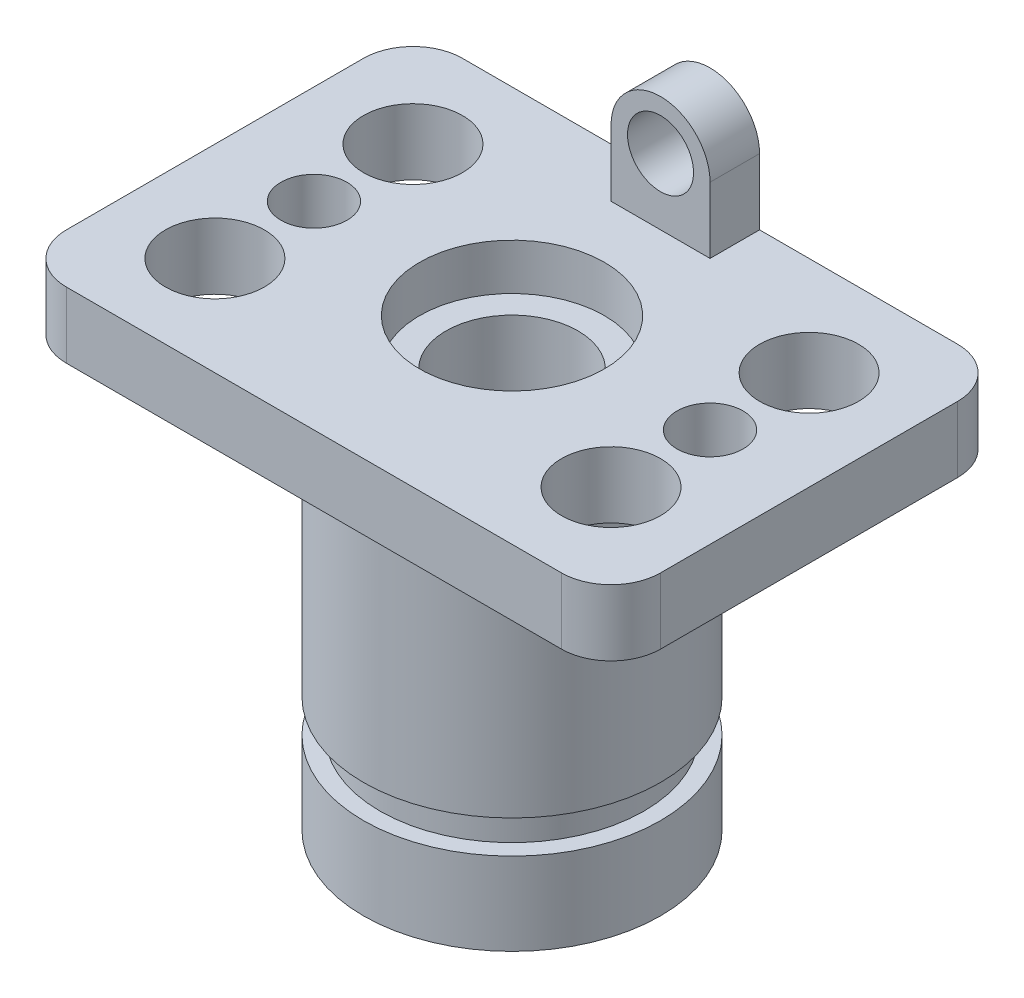
ISO-10303-21;
HEADER;
FILE_DESCRIPTION(('STEP AP214'),'2;1');
FILE_NAME('part.step','',(''),(''),'','','');
FILE_SCHEMA(('AUTOMOTIVE_DESIGN { 1 0 10303 214 1 1 1 1 }'));
ENDSEC;
DATA;
#1=APPLICATION_CONTEXT('core data for automotive mechanical design processes');
#2=APPLICATION_PROTOCOL_DEFINITION('international standard','automotive_design',2000,#1);
#3=PRODUCT_CONTEXT('',#1,'mechanical');
#4=PRODUCT('Part','Part','',(#3));
#5=PRODUCT_RELATED_PRODUCT_CATEGORY('part','',(#4));
#6=PRODUCT_DEFINITION_FORMATION('','',#4);
#7=PRODUCT_DEFINITION_CONTEXT('part definition',#1,'design');
#8=PRODUCT_DEFINITION('design','',#6,#7);
#9=PRODUCT_DEFINITION_SHAPE('','',#8);
#10=(LENGTH_UNIT() NAMED_UNIT(*) SI_UNIT(.MILLI.,.METRE.));
#11=(NAMED_UNIT(*) PLANE_ANGLE_UNIT() SI_UNIT($,.RADIAN.));
#12=(NAMED_UNIT(*) SI_UNIT($,.STERADIAN.) SOLID_ANGLE_UNIT());
#13=UNCERTAINTY_MEASURE_WITH_UNIT(LENGTH_MEASURE(1.E-05),#10,'distance_accuracy_value','');
#14=(GEOMETRIC_REPRESENTATION_CONTEXT(3) GLOBAL_UNCERTAINTY_ASSIGNED_CONTEXT((#13)) GLOBAL_UNIT_ASSIGNED_CONTEXT((#10,
#11,#12)) REPRESENTATION_CONTEXT('',''));
#15=CARTESIAN_POINT('',(0.,0.,0.));
#16=DIRECTION('',(0.,0.,1.));
#17=DIRECTION('',(1.,0.,0.));
#18=AXIS2_PLACEMENT_3D('',#15,#16,#17);
#19=CARTESIAN_POINT('',(28.,0.,0.));
#20=DIRECTION('',(0.,1.,0.));
#21=DIRECTION('',(0.,0.,1.));
#22=AXIS2_PLACEMENT_3D('',#19,#20,#21);
#23=PLANE('',#22);
#24=DIRECTION('',(0.,0.,-1.));
#25=VECTOR('',#24,1.);
#26=CARTESIAN_POINT('',(15.,0.,-45.));
#27=LINE('',#26,#25);
#28=CARTESIAN_POINT('',(15.,0.,-45.));
#29=VERTEX_POINT('',#28);
#30=CARTESIAN_POINT('',(15.,0.,-60.));
#31=VERTEX_POINT('',#30);
#32=EDGE_CURVE('E361',#29,#31,#27,.T.);
#33=ORIENTED_EDGE('',*,*,#32,.F.);
#34=DIRECTION('',(-1.,0.,0.));
#35=VECTOR('',#34,1.);
#36=CARTESIAN_POINT('',(15.,0.,-45.));
#37=LINE('',#36,#35);
#38=CARTESIAN_POINT('',(-15.,0.,-45.));
#39=VERTEX_POINT('',#38);
#40=EDGE_CURVE('E344',#29,#39,#37,.T.);
#41=ORIENTED_EDGE('',*,*,#40,.T.);
#42=DIRECTION('',(0.,0.,-1.));
#43=VECTOR('',#42,1.);
#44=CARTESIAN_POINT('',(-15.,0.,-45.));
#45=LINE('',#44,#43);
#46=CARTESIAN_POINT('',(-15.,0.,-60.));
#47=VERTEX_POINT('',#46);
#48=EDGE_CURVE('E363',#39,#47,#45,.T.);
#49=ORIENTED_EDGE('',*,*,#48,.T.);
#50=DIRECTION('',(-1.,0.,0.));
#51=VECTOR('',#50,1.);
#52=CARTESIAN_POINT('',(-75.,0.,-60.));
#53=LINE('',#52,#51);
#54=CARTESIAN_POINT('',(-75.,0.,-60.));
#55=VERTEX_POINT('',#54);
#56=EDGE_CURVE('E166',#47,#55,#53,.T.);
#57=ORIENTED_EDGE('',*,*,#56,.T.);
#58=CARTESIAN_POINT('',(-75.,0.,-45.));
#59=DIRECTION('',(0.,1.,0.));
#60=DIRECTION('',(0.,0.,-1.));
#61=AXIS2_PLACEMENT_3D('',#58,#59,#60);
#62=CIRCLE('',#61,15.);
#63=CARTESIAN_POINT('',(-90.,0.,-45.));
#64=VERTEX_POINT('',#63);
#65=EDGE_CURVE('E126',#55,#64,#62,.T.);
#66=ORIENTED_EDGE('',*,*,#65,.T.);
#67=DIRECTION('',(0.,0.,1.));
#68=VECTOR('',#67,1.);
#69=CARTESIAN_POINT('',(-90.,0.,45.));
#70=LINE('',#69,#68);
#71=CARTESIAN_POINT('',(-90.,0.,45.));
#72=VERTEX_POINT('',#71);
#73=EDGE_CURVE('E173',#64,#72,#70,.T.);
#74=ORIENTED_EDGE('',*,*,#73,.T.);
#75=CARTESIAN_POINT('',(-75.,0.,45.));
#76=DIRECTION('',(0.,1.,0.));
#77=DIRECTION('',(0.,0.,-1.));
#78=AXIS2_PLACEMENT_3D('',#75,#76,#77);
#79=CIRCLE('',#78,15.);
#80=CARTESIAN_POINT('',(-75.,0.,60.));
#81=VERTEX_POINT('',#80);
#82=EDGE_CURVE('E153',#72,#81,#79,.T.);
#83=ORIENTED_EDGE('',*,*,#82,.T.);
#84=DIRECTION('',(1.,0.,0.));
#85=VECTOR('',#84,1.);
#86=CARTESIAN_POINT('',(-75.,0.,60.));
#87=LINE('',#86,#85);
#88=CARTESIAN_POINT('',(75.,0.,60.));
#89=VERTEX_POINT('',#88);
#90=EDGE_CURVE('E156',#81,#89,#87,.T.);
#91=ORIENTED_EDGE('',*,*,#90,.T.);
#92=CARTESIAN_POINT('',(75.,0.,45.));
#93=DIRECTION('',(0.,1.,0.));
#94=DIRECTION('',(0.,0.,1.));
#95=AXIS2_PLACEMENT_3D('',#92,#93,#94);
#96=CIRCLE('',#95,15.);
#97=CARTESIAN_POINT('',(90.,0.,45.));
#98=VERTEX_POINT('',#97);
#99=EDGE_CURVE('E159',#89,#98,#96,.T.);
#100=ORIENTED_EDGE('',*,*,#99,.T.);
#101=DIRECTION('',(0.,0.,-1.));
#102=VECTOR('',#101,1.);
#103=CARTESIAN_POINT('',(90.,0.,45.));
#104=LINE('',#103,#102);
#105=CARTESIAN_POINT('',(90.,0.,-45.));
#106=VERTEX_POINT('',#105);
#107=EDGE_CURVE('E162',#98,#106,#104,.T.);
#108=ORIENTED_EDGE('',*,*,#107,.T.);
#109=CARTESIAN_POINT('',(75.,0.,-45.));
#110=DIRECTION('',(0.,1.,0.));
#111=DIRECTION('',(0.,0.,-1.));
#112=AXIS2_PLACEMENT_3D('',#109,#110,#111);
#113=CIRCLE('',#112,15.);
#114=CARTESIAN_POINT('',(75.,0.,-60.));
#115=VERTEX_POINT('',#114);
#116=EDGE_CURVE('E167',#106,#115,#113,.T.);
#117=ORIENTED_EDGE('',*,*,#116,.T.);
#118=EDGE_CURVE('E168',#115,#31,#53,.T.);
#119=ORIENTED_EDGE('',*,*,#118,.T.);
#120=EDGE_LOOP('',(#33,#41,#49,#57,#66,#74,#83,#91,#100,#108,#117,#119));
#121=FACE_BOUND('',#120,.T.);
#122=CARTESIAN_POINT('',(0.,0.,0.));
#123=DIRECTION('',(0.,-1.,0.));
#124=DIRECTION('',(0.,0.,-1.));
#125=AXIS2_PLACEMENT_3D('',#122,#123,#124);
#126=CIRCLE('',#125,28.);
#127=CARTESIAN_POINT('',(0.,0.,-28.));
#128=VERTEX_POINT('',#127);
#129=EDGE_CURVE('E178',#128,#128,#126,.T.);
#130=ORIENTED_EDGE('',*,*,#129,.T.);
#131=EDGE_LOOP('',(#130));
#132=FACE_BOUND('',#131,.T.);
#133=CARTESIAN_POINT('',(60.,0.,-30.));
#134=DIRECTION('',(0.,1.,0.));
#135=DIRECTION('',(0.,0.,-1.));
#136=AXIS2_PLACEMENT_3D('',#133,#134,#135);
#137=CIRCLE('',#136,15.);
#138=CARTESIAN_POINT('',(60.,0.,-45.));
#139=VERTEX_POINT('',#138);
#140=EDGE_CURVE('E359',#139,#139,#137,.T.);
#141=ORIENTED_EDGE('',*,*,#140,.F.);
#142=EDGE_LOOP('',(#141));
#143=FACE_BOUND('',#142,.T.);
#144=CARTESIAN_POINT('',(60.,0.,0.));
#145=DIRECTION('',(0.,1.,0.));
#146=DIRECTION('',(0.,0.,-1.));
#147=AXIS2_PLACEMENT_3D('',#144,#145,#146);
#148=CIRCLE('',#147,9.99999999999999);
#149=CARTESIAN_POINT('',(60.,0.,-9.99999999999999));
#150=VERTEX_POINT('',#149);
#151=EDGE_CURVE('E371',#150,#150,#148,.T.);
#152=ORIENTED_EDGE('',*,*,#151,.F.);
#153=EDGE_LOOP('',(#152));
#154=FACE_BOUND('',#153,.T.);
#155=CARTESIAN_POINT('',(60.,0.,30.));
#156=DIRECTION('',(0.,1.,0.));
#157=DIRECTION('',(0.,0.,-1.));
#158=AXIS2_PLACEMENT_3D('',#155,#156,#157);
#159=CIRCLE('',#158,15.);
#160=CARTESIAN_POINT('',(60.,0.,15.));
#161=VERTEX_POINT('',#160);
#162=EDGE_CURVE('E380',#161,#161,#159,.T.);
#163=ORIENTED_EDGE('',*,*,#162,.F.);
#164=EDGE_LOOP('',(#163));
#165=FACE_BOUND('',#164,.T.);
#166=CARTESIAN_POINT('',(-60.,0.,-30.));
#167=DIRECTION('',(0.,1.,0.));
#168=DIRECTION('',(0.,0.,1.));
#169=AXIS2_PLACEMENT_3D('',#166,#167,#168);
#170=CIRCLE('',#169,15.);
#171=CARTESIAN_POINT('',(-60.,0.,-15.));
#172=VERTEX_POINT('',#171);
#173=EDGE_CURVE('E382',#172,#172,#170,.T.);
#174=ORIENTED_EDGE('',*,*,#173,.F.);
#175=EDGE_LOOP('',(#174));
#176=FACE_BOUND('',#175,.T.);
#177=CARTESIAN_POINT('',(-60.,0.,0.));
#178=DIRECTION('',(0.,1.,0.));
#179=DIRECTION('',(0.,0.,1.));
#180=AXIS2_PLACEMENT_3D('',#177,#178,#179);
#181=CIRCLE('',#180,9.99999999999999);
#182=CARTESIAN_POINT('',(-60.,0.,9.99999999999999));
#183=VERTEX_POINT('',#182);
#184=EDGE_CURVE('E386',#183,#183,#181,.T.);
#185=ORIENTED_EDGE('',*,*,#184,.F.);
#186=EDGE_LOOP('',(#185));
#187=FACE_BOUND('',#186,.T.);
#188=CARTESIAN_POINT('',(-60.,0.,30.));
#189=DIRECTION('',(0.,1.,0.));
#190=DIRECTION('',(0.,0.,1.));
#191=AXIS2_PLACEMENT_3D('',#188,#189,#190);
#192=CIRCLE('',#191,15.);
#193=CARTESIAN_POINT('',(-60.,0.,45.));
#194=VERTEX_POINT('',#193);
#195=EDGE_CURVE('E394',#194,#194,#192,.T.);
#196=ORIENTED_EDGE('',*,*,#195,.F.);
#197=EDGE_LOOP('',(#196));
#198=FACE_BOUND('',#197,.T.);
#199=ADVANCED_FACE('F39',(#121,#132,#143,#154,#165,#176,#187,#198),#23,.T.);
#200=CARTESIAN_POINT('',(0.,-88.6363199538716,0.));
#201=DIRECTION('',(0.,-1.,0.));
#202=DIRECTION('',(0.,0.,-1.));
#203=AXIS2_PLACEMENT_3D('',#200,#201,#202);
#204=CYLINDRICAL_SURFACE('',#203,45.);
#205=CARTESIAN_POINT('',(0.,-20.,0.));
#206=DIRECTION('',(0.,-1.,0.));
#207=DIRECTION('',(0.,0.,-1.));
#208=AXIS2_PLACEMENT_3D('',#205,#206,#207);
#209=CIRCLE('',#208,45.);
#210=CARTESIAN_POINT('',(0.,-20.,-45.));
#211=VERTEX_POINT('',#210);
#212=EDGE_CURVE('E11',#211,#211,#209,.F.);
#213=ORIENTED_EDGE('',*,*,#212,.F.);
#214=EDGE_LOOP('',(#213));
#215=FACE_BOUND('',#214,.T.);
#216=CARTESIAN_POINT('',(0.,-100.,0.));
#217=DIRECTION('',(0.,-1.,0.));
#218=DIRECTION('',(0.,0.,-1.));
#219=AXIS2_PLACEMENT_3D('',#216,#217,#218);
#220=CIRCLE('',#219,45.);
#221=CARTESIAN_POINT('',(0.,-100.,-45.));
#222=VERTEX_POINT('',#221);
#223=EDGE_CURVE('E46',#222,#222,#220,.T.);
#224=ORIENTED_EDGE('',*,*,#223,.F.);
#225=EDGE_LOOP('',(#224));
#226=FACE_BOUND('',#225,.T.);
#227=ADVANCED_FACE('F220',(#215,#226),#204,.T.);
#228=CARTESIAN_POINT('',(45.,-100.,0.));
#229=DIRECTION('',(0.,-1.,0.));
#230=DIRECTION('',(0.,0.,-1.));
#231=AXIS2_PLACEMENT_3D('',#228,#229,#230);
#232=PLANE('',#231);
#233=ORIENTED_EDGE('',*,*,#223,.T.);
#234=EDGE_LOOP('',(#233));
#235=FACE_BOUND('',#234,.T.);
#236=CARTESIAN_POINT('',(0.,-100.,0.));
#237=DIRECTION('',(0.,-1.,0.));
#238=DIRECTION('',(0.,0.,-1.));
#239=AXIS2_PLACEMENT_3D('',#236,#237,#238);
#240=CIRCLE('',#239,40.);
#241=CARTESIAN_POINT('',(0.,-100.,-40.));
#242=VERTEX_POINT('',#241);
#243=EDGE_CURVE('E207',#242,#242,#240,.T.);
#244=ORIENTED_EDGE('',*,*,#243,.F.);
#245=EDGE_LOOP('',(#244));
#246=FACE_BOUND('',#245,.T.);
#247=ADVANCED_FACE('F212',(#235,#246),#232,.T.);
#248=CARTESIAN_POINT('',(0.,-88.6363199538716,0.));
#249=DIRECTION('',(0.,-1.,0.));
#250=DIRECTION('',(0.,0.,-1.));
#251=AXIS2_PLACEMENT_3D('',#248,#249,#250);
#252=CYLINDRICAL_SURFACE('',#251,40.);
#253=ORIENTED_EDGE('',*,*,#243,.T.);
#254=EDGE_LOOP('',(#253));
#255=FACE_BOUND('',#254,.T.);
#256=CARTESIAN_POINT('',(0.,-110.,0.));
#257=DIRECTION('',(0.,-1.,0.));
#258=DIRECTION('',(0.,0.,-1.));
#259=AXIS2_PLACEMENT_3D('',#256,#257,#258);
#260=CIRCLE('',#259,40.);
#261=CARTESIAN_POINT('',(0.,-110.,-40.));
#262=VERTEX_POINT('',#261);
#263=EDGE_CURVE('E206',#262,#262,#260,.T.);
#264=ORIENTED_EDGE('',*,*,#263,.F.);
#265=EDGE_LOOP('',(#264));
#266=FACE_BOUND('',#265,.T.);
#267=ADVANCED_FACE('F223',(#255,#266),#252,.T.);
#268=CARTESIAN_POINT('',(40.,-110.,0.));
#269=DIRECTION('',(0.,1.,0.));
#270=DIRECTION('',(0.,0.,1.));
#271=AXIS2_PLACEMENT_3D('',#268,#269,#270);
#272=PLANE('',#271);
#273=ORIENTED_EDGE('',*,*,#263,.T.);
#274=EDGE_LOOP('',(#273));
#275=FACE_BOUND('',#274,.T.);
#276=CARTESIAN_POINT('',(0.,-110.,0.));
#277=DIRECTION('',(0.,-1.,0.));
#278=DIRECTION('',(0.,0.,-1.));
#279=AXIS2_PLACEMENT_3D('',#276,#277,#278);
#280=CIRCLE('',#279,45.);
#281=CARTESIAN_POINT('',(0.,-110.,-45.));
#282=VERTEX_POINT('',#281);
#283=EDGE_CURVE('E201',#282,#282,#280,.T.);
#284=ORIENTED_EDGE('',*,*,#283,.F.);
#285=EDGE_LOOP('',(#284));
#286=FACE_BOUND('',#285,.T.);
#287=ADVANCED_FACE('F232',(#275,#286),#272,.T.);
#288=CARTESIAN_POINT('',(0.,-88.6363199538716,0.));
#289=DIRECTION('',(0.,-1.,0.));
#290=DIRECTION('',(0.,0.,-1.));
#291=AXIS2_PLACEMENT_3D('',#288,#289,#290);
#292=CYLINDRICAL_SURFACE('',#291,45.);
#293=ORIENTED_EDGE('',*,*,#283,.T.);
#294=EDGE_LOOP('',(#293));
#295=FACE_BOUND('',#294,.T.);
#296=CARTESIAN_POINT('',(0.,-135.,0.));
#297=DIRECTION('',(0.,-1.,0.));
#298=DIRECTION('',(0.,0.,-1.));
#299=AXIS2_PLACEMENT_3D('',#296,#297,#298);
#300=CIRCLE('',#299,45.);
#301=CARTESIAN_POINT('',(0.,-135.,-45.));
#302=VERTEX_POINT('',#301);
#303=EDGE_CURVE('E199',#302,#302,#300,.T.);
#304=ORIENTED_EDGE('',*,*,#303,.F.);
#305=EDGE_LOOP('',(#304));
#306=FACE_BOUND('',#305,.T.);
#307=ADVANCED_FACE('F240',(#295,#306),#292,.T.);
#308=CARTESIAN_POINT('',(45.,-135.,0.));
#309=DIRECTION('',(0.,-1.,0.));
#310=DIRECTION('',(0.,0.,-1.));
#311=AXIS2_PLACEMENT_3D('',#308,#309,#310);
#312=PLANE('',#311);
#313=ORIENTED_EDGE('',*,*,#303,.T.);
#314=EDGE_LOOP('',(#313));
#315=FACE_BOUND('',#314,.T.);
#316=CARTESIAN_POINT('',(0.,-135.,0.));
#317=DIRECTION('',(0.,-1.,0.));
#318=DIRECTION('',(0.,0.,-1.));
#319=AXIS2_PLACEMENT_3D('',#316,#317,#318);
#320=CIRCLE('',#319,20.);
#321=CARTESIAN_POINT('',(0.,-135.,-20.));
#322=VERTEX_POINT('',#321);
#323=EDGE_CURVE('E197',#322,#322,#320,.T.);
#324=ORIENTED_EDGE('',*,*,#323,.F.);
#325=EDGE_LOOP('',(#324));
#326=FACE_BOUND('',#325,.T.);
#327=ADVANCED_FACE('F241',(#315,#326),#312,.T.);
#328=CARTESIAN_POINT('',(0.,-88.6363199538716,0.));
#329=DIRECTION('',(0.,-1.,0.));
#330=DIRECTION('',(0.,0.,-1.));
#331=AXIS2_PLACEMENT_3D('',#328,#329,#330);
#332=CYLINDRICAL_SURFACE('',#331,20.);
#333=ORIENTED_EDGE('',*,*,#323,.T.);
#334=EDGE_LOOP('',(#333));
#335=FACE_BOUND('',#334,.T.);
#336=CARTESIAN_POINT('',(0.,-14.,0.));
#337=DIRECTION('',(0.,-1.,0.));
#338=DIRECTION('',(0.,0.,-1.));
#339=AXIS2_PLACEMENT_3D('',#336,#337,#338);
#340=CIRCLE('',#339,20.);
#341=CARTESIAN_POINT('',(0.,-14.,-20.));
#342=VERTEX_POINT('',#341);
#343=EDGE_CURVE('E193',#342,#342,#340,.T.);
#344=ORIENTED_EDGE('',*,*,#343,.F.);
#345=EDGE_LOOP('',(#344));
#346=FACE_BOUND('',#345,.T.);
#347=ADVANCED_FACE('F244',(#335,#346),#332,.F.);
#348=CARTESIAN_POINT('',(20.,-14.,0.));
#349=DIRECTION('',(0.,1.,0.));
#350=DIRECTION('',(0.,0.,1.));
#351=AXIS2_PLACEMENT_3D('',#348,#349,#350);
#352=PLANE('',#351);
#353=ORIENTED_EDGE('',*,*,#343,.T.);
#354=EDGE_LOOP('',(#353));
#355=FACE_BOUND('',#354,.T.);
#356=CARTESIAN_POINT('',(0.,-14.,0.));
#357=DIRECTION('',(0.,-1.,0.));
#358=DIRECTION('',(0.,0.,-1.));
#359=AXIS2_PLACEMENT_3D('',#356,#357,#358);
#360=CIRCLE('',#359,28.);
#361=CARTESIAN_POINT('',(0.,-14.,-28.));
#362=VERTEX_POINT('',#361);
#363=EDGE_CURVE('E191',#362,#362,#360,.T.);
#364=ORIENTED_EDGE('',*,*,#363,.F.);
#365=EDGE_LOOP('',(#364));
#366=FACE_BOUND('',#365,.T.);
#367=ADVANCED_FACE('F248',(#355,#366),#352,.T.);
#368=CARTESIAN_POINT('',(0.,-88.6363199538716,0.));
#369=DIRECTION('',(0.,-1.,0.));
#370=DIRECTION('',(0.,0.,-1.));
#371=AXIS2_PLACEMENT_3D('',#368,#369,#370);
#372=CYLINDRICAL_SURFACE('',#371,28.);
#373=ORIENTED_EDGE('',*,*,#363,.T.);
#374=EDGE_LOOP('',(#373));
#375=FACE_BOUND('',#374,.T.);
#376=ORIENTED_EDGE('',*,*,#129,.F.);
#377=EDGE_LOOP('',(#376));
#378=FACE_BOUND('',#377,.T.);
#379=ADVANCED_FACE('F251',(#375,#378),#372,.F.);
#380=CARTESIAN_POINT('',(-75.,-20.,45.));
#381=DIRECTION('',(0.,1.,0.));
#382=DIRECTION('',(0.,0.,1.));
#383=AXIS2_PLACEMENT_3D('',#380,#381,#382);
#384=CYLINDRICAL_SURFACE('',#383,15.);
#385=ORIENTED_EDGE('',*,*,#82,.F.);
#386=DIRECTION('',(0.,1.,0.));
#387=VECTOR('',#386,1.);
#388=CARTESIAN_POINT('',(-90.,-20.,45.));
#389=LINE('',#388,#387);
#390=CARTESIAN_POINT('',(-90.,-20.,45.));
#391=VERTEX_POINT('',#390);
#392=EDGE_CURVE('E65',#391,#72,#389,.T.);
#393=ORIENTED_EDGE('',*,*,#392,.F.);
#394=CARTESIAN_POINT('',(-75.,-20.,45.));
#395=DIRECTION('',(0.,1.,0.));
#396=DIRECTION('',(0.,0.,-1.));
#397=AXIS2_PLACEMENT_3D('',#394,#395,#396);
#398=CIRCLE('',#397,15.);
#399=CARTESIAN_POINT('',(-75.,-20.,60.));
#400=VERTEX_POINT('',#399);
#401=EDGE_CURVE('E180',#391,#400,#398,.T.);
#402=ORIENTED_EDGE('',*,*,#401,.T.);
#403=DIRECTION('',(0.,1.,0.));
#404=VECTOR('',#403,1.);
#405=CARTESIAN_POINT('',(-75.,-20.,60.));
#406=LINE('',#405,#404);
#407=EDGE_CURVE('E101',#400,#81,#406,.T.);
#408=ORIENTED_EDGE('',*,*,#407,.T.);
#409=EDGE_LOOP('',(#385,#393,#402,#408));
#410=FACE_BOUND('',#409,.T.);
#411=ADVANCED_FACE('F258',(#410),#384,.T.);
#412=CARTESIAN_POINT('',(-90.,-20.,45.));
#413=DIRECTION('',(-1.,0.,0.));
#414=DIRECTION('',(0.,0.,1.));
#415=AXIS2_PLACEMENT_3D('',#412,#413,#414);
#416=PLANE('',#415);
#417=ORIENTED_EDGE('',*,*,#73,.F.);
#418=DIRECTION('',(0.,1.,0.));
#419=VECTOR('',#418,1.);
#420=CARTESIAN_POINT('',(-90.,-20.,-45.));
#421=LINE('',#420,#419);
#422=CARTESIAN_POINT('',(-90.,-20.,-45.));
#423=VERTEX_POINT('',#422);
#424=EDGE_CURVE('E135',#423,#64,#421,.T.);
#425=ORIENTED_EDGE('',*,*,#424,.F.);
#426=DIRECTION('',(0.,0.,1.));
#427=VECTOR('',#426,1.);
#428=CARTESIAN_POINT('',(-90.,-20.,45.));
#429=LINE('',#428,#427);
#430=EDGE_CURVE('E143',#423,#391,#429,.T.);
#431=ORIENTED_EDGE('',*,*,#430,.T.);
#432=ORIENTED_EDGE('',*,*,#392,.T.);
#433=EDGE_LOOP('',(#417,#425,#431,#432));
#434=FACE_BOUND('',#433,.T.);
#435=ADVANCED_FACE('F259',(#434),#416,.T.);
#436=CARTESIAN_POINT('',(-75.,-20.,-45.));
#437=DIRECTION('',(0.,1.,0.));
#438=DIRECTION('',(0.,0.,1.));
#439=AXIS2_PLACEMENT_3D('',#436,#437,#438);
#440=CYLINDRICAL_SURFACE('',#439,15.);
#441=ORIENTED_EDGE('',*,*,#65,.F.);
#442=DIRECTION('',(0.,1.,0.));
#443=VECTOR('',#442,1.);
#444=CARTESIAN_POINT('',(-75.,-20.,-60.));
#445=LINE('',#444,#443);
#446=CARTESIAN_POINT('',(-75.,-20.,-60.));
#447=VERTEX_POINT('',#446);
#448=EDGE_CURVE('E125',#447,#55,#445,.T.);
#449=ORIENTED_EDGE('',*,*,#448,.F.);
#450=CARTESIAN_POINT('',(-75.,-20.,-45.));
#451=DIRECTION('',(0.,1.,0.));
#452=DIRECTION('',(0.,0.,-1.));
#453=AXIS2_PLACEMENT_3D('',#450,#451,#452);
#454=CIRCLE('',#453,15.);
#455=EDGE_CURVE('E124',#447,#423,#454,.T.);
#456=ORIENTED_EDGE('',*,*,#455,.T.);
#457=ORIENTED_EDGE('',*,*,#424,.T.);
#458=EDGE_LOOP('',(#441,#449,#456,#457));
#459=FACE_BOUND('',#458,.T.);
#460=ADVANCED_FACE('F123',(#459),#440,.T.);
#461=CARTESIAN_POINT('',(-75.,-20.,-60.));
#462=DIRECTION('',(0.,0.,-1.));
#463=DIRECTION('',(-1.,0.,0.));
#464=AXIS2_PLACEMENT_3D('',#461,#462,#463);
#465=PLANE('',#464);
#466=ORIENTED_EDGE('',*,*,#118,.F.);
#467=DIRECTION('',(0.,1.,0.));
#468=VECTOR('',#467,1.);
#469=CARTESIAN_POINT('',(75.,-20.,-60.));
#470=LINE('',#469,#468);
#471=CARTESIAN_POINT('',(75.,-20.,-60.));
#472=VERTEX_POINT('',#471);
#473=EDGE_CURVE('E132',#472,#115,#470,.T.);
#474=ORIENTED_EDGE('',*,*,#473,.F.);
#475=DIRECTION('',(-1.,0.,0.));
#476=VECTOR('',#475,1.);
#477=CARTESIAN_POINT('',(-75.,-20.,-60.));
#478=LINE('',#477,#476);
#479=EDGE_CURVE('E138',#472,#447,#478,.T.);
#480=ORIENTED_EDGE('',*,*,#479,.T.);
#481=ORIENTED_EDGE('',*,*,#448,.T.);
#482=ORIENTED_EDGE('',*,*,#56,.F.);
#483=DIRECTION('',(0.,1.,0.));
#484=VECTOR('',#483,1.);
#485=CARTESIAN_POINT('',(-15.,0.,-60.));
#486=LINE('',#485,#484);
#487=CARTESIAN_POINT('',(-15.,20.,-60.));
#488=VERTEX_POINT('',#487);
#489=EDGE_CURVE('E52',#47,#488,#486,.T.);
#490=ORIENTED_EDGE('',*,*,#489,.T.);
#491=CARTESIAN_POINT('',(0.,20.,-60.));
#492=DIRECTION('',(0.,0.,-1.));
#493=DIRECTION('',(-1.,0.,0.));
#494=AXIS2_PLACEMENT_3D('',#491,#492,#493);
#495=CIRCLE('',#494,15.);
#496=CARTESIAN_POINT('',(15.,20.,-60.));
#497=VERTEX_POINT('',#496);
#498=EDGE_CURVE('E336',#488,#497,#495,.T.);
#499=ORIENTED_EDGE('',*,*,#498,.T.);
#500=DIRECTION('',(0.,-1.,0.));
#501=VECTOR('',#500,1.);
#502=CARTESIAN_POINT('',(15.,20.,-60.));
#503=LINE('',#502,#501);
#504=EDGE_CURVE('E353',#497,#31,#503,.T.);
#505=ORIENTED_EDGE('',*,*,#504,.T.);
#506=EDGE_LOOP('',(#466,#474,#480,#481,#482,#490,#499,#505));
#507=FACE_BOUND('',#506,.T.);
#508=CARTESIAN_POINT('',(0.,20.,-60.));
#509=DIRECTION('',(0.,0.,-1.));
#510=DIRECTION('',(-1.,0.,0.));
#511=AXIS2_PLACEMENT_3D('',#508,#509,#510);
#512=CIRCLE('',#511,10.);
#513=CARTESIAN_POINT('',(-10.,20.,-60.));
#514=VERTEX_POINT('',#513);
#515=EDGE_CURVE('E331',#514,#514,#512,.T.);
#516=ORIENTED_EDGE('',*,*,#515,.F.);
#517=EDGE_LOOP('',(#516));
#518=FACE_BOUND('',#517,.T.);
#519=ADVANCED_FACE('F145',(#507,#518),#465,.T.);
#520=CARTESIAN_POINT('',(75.,-20.,-45.));
#521=DIRECTION('',(0.,1.,0.));
#522=DIRECTION('',(0.,0.,1.));
#523=AXIS2_PLACEMENT_3D('',#520,#521,#522);
#524=CYLINDRICAL_SURFACE('',#523,15.);
#525=ORIENTED_EDGE('',*,*,#116,.F.);
#526=DIRECTION('',(0.,1.,0.));
#527=VECTOR('',#526,1.);
#528=CARTESIAN_POINT('',(90.,-20.,-45.));
#529=LINE('',#528,#527);
#530=CARTESIAN_POINT('',(90.,-20.,-45.));
#531=VERTEX_POINT('',#530);
#532=EDGE_CURVE('E185',#531,#106,#529,.T.);
#533=ORIENTED_EDGE('',*,*,#532,.F.);
#534=CARTESIAN_POINT('',(75.,-20.,-45.));
#535=DIRECTION('',(0.,1.,0.));
#536=DIRECTION('',(0.,0.,-1.));
#537=AXIS2_PLACEMENT_3D('',#534,#535,#536);
#538=CIRCLE('',#537,15.);
#539=EDGE_CURVE('E148',#531,#472,#538,.T.);
#540=ORIENTED_EDGE('',*,*,#539,.T.);
#541=ORIENTED_EDGE('',*,*,#473,.T.);
#542=EDGE_LOOP('',(#525,#533,#540,#541));
#543=FACE_BOUND('',#542,.T.);
#544=ADVANCED_FACE('F269',(#543),#524,.T.);
#545=CARTESIAN_POINT('',(90.,-20.,45.));
#546=DIRECTION('',(1.,0.,0.));
#547=DIRECTION('',(0.,0.,-1.));
#548=AXIS2_PLACEMENT_3D('',#545,#546,#547);
#549=PLANE('',#548);
#550=ORIENTED_EDGE('',*,*,#107,.F.);
#551=DIRECTION('',(0.,1.,0.));
#552=VECTOR('',#551,1.);
#553=CARTESIAN_POINT('',(90.,-20.,45.));
#554=LINE('',#553,#552);
#555=CARTESIAN_POINT('',(90.,-20.,45.));
#556=VERTEX_POINT('',#555);
#557=EDGE_CURVE('E184',#556,#98,#554,.T.);
#558=ORIENTED_EDGE('',*,*,#557,.F.);
#559=DIRECTION('',(0.,0.,-1.));
#560=VECTOR('',#559,1.);
#561=CARTESIAN_POINT('',(90.,-20.,45.));
#562=LINE('',#561,#560);
#563=EDGE_CURVE('E146',#556,#531,#562,.T.);
#564=ORIENTED_EDGE('',*,*,#563,.T.);
#565=ORIENTED_EDGE('',*,*,#532,.T.);
#566=EDGE_LOOP('',(#550,#558,#564,#565));
#567=FACE_BOUND('',#566,.T.);
#568=ADVANCED_FACE('F266',(#567),#549,.T.);
#569=CARTESIAN_POINT('',(75.,-20.,45.));
#570=DIRECTION('',(0.,1.,0.));
#571=DIRECTION('',(0.,0.,1.));
#572=AXIS2_PLACEMENT_3D('',#569,#570,#571);
#573=CYLINDRICAL_SURFACE('',#572,15.);
#574=ORIENTED_EDGE('',*,*,#99,.F.);
#575=DIRECTION('',(0.,1.,0.));
#576=VECTOR('',#575,1.);
#577=CARTESIAN_POINT('',(75.,-20.,60.));
#578=LINE('',#577,#576);
#579=CARTESIAN_POINT('',(75.,-20.,60.));
#580=VERTEX_POINT('',#579);
#581=EDGE_CURVE('E186',#580,#89,#578,.T.);
#582=ORIENTED_EDGE('',*,*,#581,.F.);
#583=CARTESIAN_POINT('',(75.,-20.,45.));
#584=DIRECTION('',(0.,1.,0.));
#585=DIRECTION('',(0.,0.,1.));
#586=AXIS2_PLACEMENT_3D('',#583,#584,#585);
#587=CIRCLE('',#586,15.);
#588=EDGE_CURVE('E403',#580,#556,#587,.T.);
#589=ORIENTED_EDGE('',*,*,#588,.T.);
#590=ORIENTED_EDGE('',*,*,#557,.T.);
#591=EDGE_LOOP('',(#574,#582,#589,#590));
#592=FACE_BOUND('',#591,.T.);
#593=ADVANCED_FACE('F263',(#592),#573,.T.);
#594=CARTESIAN_POINT('',(-75.,-20.,60.));
#595=DIRECTION('',(0.,0.,1.));
#596=DIRECTION('',(1.,0.,0.));
#597=AXIS2_PLACEMENT_3D('',#594,#595,#596);
#598=PLANE('',#597);
#599=ORIENTED_EDGE('',*,*,#90,.F.);
#600=ORIENTED_EDGE('',*,*,#407,.F.);
#601=DIRECTION('',(1.,0.,0.));
#602=VECTOR('',#601,1.);
#603=CARTESIAN_POINT('',(-75.,-20.,60.));
#604=LINE('',#603,#602);
#605=EDGE_CURVE('E401',#400,#580,#604,.T.);
#606=ORIENTED_EDGE('',*,*,#605,.T.);
#607=ORIENTED_EDGE('',*,*,#581,.T.);
#608=EDGE_LOOP('',(#599,#600,#606,#607));
#609=FACE_BOUND('',#608,.T.);
#610=ADVANCED_FACE('F257',(#609),#598,.T.);
#611=CARTESIAN_POINT('',(-75.,-20.,45.));
#612=DIRECTION('',(0.,-1.,0.));
#613=DIRECTION('',(0.,0.,-1.));
#614=AXIS2_PLACEMENT_3D('',#611,#612,#613);
#615=PLANE('',#614);
#616=ORIENTED_EDGE('',*,*,#212,.T.);
#617=EDGE_LOOP('',(#616));
#618=FACE_BOUND('',#617,.T.);
#619=CARTESIAN_POINT('',(60.,-20.,-30.));
#620=DIRECTION('',(0.,1.,0.));
#621=DIRECTION('',(0.,0.,-1.));
#622=AXIS2_PLACEMENT_3D('',#619,#620,#621);
#623=CIRCLE('',#622,15.);
#624=CARTESIAN_POINT('',(60.,-20.,-45.));
#625=VERTEX_POINT('',#624);
#626=EDGE_CURVE('E366',#625,#625,#623,.T.);
#627=ORIENTED_EDGE('',*,*,#626,.T.);
#628=EDGE_LOOP('',(#627));
#629=FACE_BOUND('',#628,.T.);
#630=CARTESIAN_POINT('',(60.,-20.,0.));
#631=DIRECTION('',(0.,1.,0.));
#632=DIRECTION('',(0.,0.,-1.));
#633=AXIS2_PLACEMENT_3D('',#630,#631,#632);
#634=CIRCLE('',#633,9.99999999999999);
#635=CARTESIAN_POINT('',(60.,-20.,-9.99999999999999));
#636=VERTEX_POINT('',#635);
#637=EDGE_CURVE('E372',#636,#636,#634,.T.);
#638=ORIENTED_EDGE('',*,*,#637,.T.);
#639=EDGE_LOOP('',(#638));
#640=FACE_BOUND('',#639,.T.);
#641=CARTESIAN_POINT('',(60.,-20.,30.));
#642=DIRECTION('',(0.,1.,0.));
#643=DIRECTION('',(0.,0.,-1.));
#644=AXIS2_PLACEMENT_3D('',#641,#642,#643);
#645=CIRCLE('',#644,15.);
#646=CARTESIAN_POINT('',(60.,-20.,15.));
#647=VERTEX_POINT('',#646);
#648=EDGE_CURVE('E379',#647,#647,#645,.T.);
#649=ORIENTED_EDGE('',*,*,#648,.T.);
#650=EDGE_LOOP('',(#649));
#651=FACE_BOUND('',#650,.T.);
#652=CARTESIAN_POINT('',(-60.,-20.,-30.));
#653=DIRECTION('',(0.,1.,0.));
#654=DIRECTION('',(0.,0.,1.));
#655=AXIS2_PLACEMENT_3D('',#652,#653,#654);
#656=CIRCLE('',#655,15.);
#657=CARTESIAN_POINT('',(-60.,-20.,-15.));
#658=VERTEX_POINT('',#657);
#659=EDGE_CURVE('E387',#658,#658,#656,.T.);
#660=ORIENTED_EDGE('',*,*,#659,.T.);
#661=EDGE_LOOP('',(#660));
#662=FACE_BOUND('',#661,.T.);
#663=CARTESIAN_POINT('',(-60.,-20.,0.));
#664=DIRECTION('',(0.,1.,0.));
#665=DIRECTION('',(0.,0.,1.));
#666=AXIS2_PLACEMENT_3D('',#663,#664,#665);
#667=CIRCLE('',#666,9.99999999999999);
#668=CARTESIAN_POINT('',(-60.,-20.,9.99999999999999));
#669=VERTEX_POINT('',#668);
#670=EDGE_CURVE('E395',#669,#669,#667,.T.);
#671=ORIENTED_EDGE('',*,*,#670,.T.);
#672=EDGE_LOOP('',(#671));
#673=FACE_BOUND('',#672,.T.);
#674=CARTESIAN_POINT('',(-60.,-20.,30.));
#675=DIRECTION('',(0.,1.,0.));
#676=DIRECTION('',(0.,0.,1.));
#677=AXIS2_PLACEMENT_3D('',#674,#675,#676);
#678=CIRCLE('',#677,15.);
#679=CARTESIAN_POINT('',(-60.,-20.,45.));
#680=VERTEX_POINT('',#679);
#681=EDGE_CURVE('E160',#680,#680,#678,.T.);
#682=ORIENTED_EDGE('',*,*,#681,.T.);
#683=EDGE_LOOP('',(#682));
#684=FACE_BOUND('',#683,.T.);
#685=ORIENTED_EDGE('',*,*,#401,.F.);
#686=ORIENTED_EDGE('',*,*,#430,.F.);
#687=ORIENTED_EDGE('',*,*,#455,.F.);
#688=ORIENTED_EDGE('',*,*,#479,.F.);
#689=ORIENTED_EDGE('',*,*,#539,.F.);
#690=ORIENTED_EDGE('',*,*,#563,.F.);
#691=ORIENTED_EDGE('',*,*,#588,.F.);
#692=ORIENTED_EDGE('',*,*,#605,.F.);
#693=EDGE_LOOP('',(#685,#686,#687,#688,#689,#690,#691,#692));
#694=FACE_BOUND('',#693,.T.);
#695=ADVANCED_FACE('F140',(#618,#629,#640,#651,#662,#673,#684,#694),#615,.T.);
#696=CARTESIAN_POINT('',(-60.,-20.,30.));
#697=DIRECTION('',(0.,1.,0.));
#698=DIRECTION('',(0.,0.,1.));
#699=AXIS2_PLACEMENT_3D('',#696,#697,#698);
#700=CYLINDRICAL_SURFACE('',#699,15.);
#701=ORIENTED_EDGE('',*,*,#681,.F.);
#702=EDGE_LOOP('',(#701));
#703=FACE_BOUND('',#702,.T.);
#704=ORIENTED_EDGE('',*,*,#195,.T.);
#705=EDGE_LOOP('',(#704));
#706=FACE_BOUND('',#705,.T.);
#707=ADVANCED_FACE('F282',(#703,#706),#700,.F.);
#708=CARTESIAN_POINT('',(-60.,-20.,0.));
#709=DIRECTION('',(0.,1.,0.));
#710=DIRECTION('',(0.,0.,1.));
#711=AXIS2_PLACEMENT_3D('',#708,#709,#710);
#712=CYLINDRICAL_SURFACE('',#711,9.99999999999999);
#713=ORIENTED_EDGE('',*,*,#670,.F.);
#714=EDGE_LOOP('',(#713));
#715=FACE_BOUND('',#714,.T.);
#716=ORIENTED_EDGE('',*,*,#184,.T.);
#717=EDGE_LOOP('',(#716));
#718=FACE_BOUND('',#717,.T.);
#719=ADVANCED_FACE('F290',(#715,#718),#712,.F.);
#720=CARTESIAN_POINT('',(-60.,-20.,-30.));
#721=DIRECTION('',(0.,1.,0.));
#722=DIRECTION('',(0.,0.,1.));
#723=AXIS2_PLACEMENT_3D('',#720,#721,#722);
#724=CYLINDRICAL_SURFACE('',#723,15.);
#725=ORIENTED_EDGE('',*,*,#659,.F.);
#726=EDGE_LOOP('',(#725));
#727=FACE_BOUND('',#726,.T.);
#728=ORIENTED_EDGE('',*,*,#173,.T.);
#729=EDGE_LOOP('',(#728));
#730=FACE_BOUND('',#729,.T.);
#731=ADVANCED_FACE('F292',(#727,#730),#724,.F.);
#732=CARTESIAN_POINT('',(60.,-20.,30.));
#733=DIRECTION('',(0.,1.,0.));
#734=DIRECTION('',(0.,0.,1.));
#735=AXIS2_PLACEMENT_3D('',#732,#733,#734);
#736=CYLINDRICAL_SURFACE('',#735,15.);
#737=ORIENTED_EDGE('',*,*,#648,.F.);
#738=EDGE_LOOP('',(#737));
#739=FACE_BOUND('',#738,.T.);
#740=ORIENTED_EDGE('',*,*,#162,.T.);
#741=EDGE_LOOP('',(#740));
#742=FACE_BOUND('',#741,.T.);
#743=ADVANCED_FACE('F293',(#739,#742),#736,.F.);
#744=CARTESIAN_POINT('',(60.,-20.,0.));
#745=DIRECTION('',(0.,1.,0.));
#746=DIRECTION('',(0.,0.,1.));
#747=AXIS2_PLACEMENT_3D('',#744,#745,#746);
#748=CYLINDRICAL_SURFACE('',#747,9.99999999999999);
#749=ORIENTED_EDGE('',*,*,#637,.F.);
#750=EDGE_LOOP('',(#749));
#751=FACE_BOUND('',#750,.T.);
#752=ORIENTED_EDGE('',*,*,#151,.T.);
#753=EDGE_LOOP('',(#752));
#754=FACE_BOUND('',#753,.T.);
#755=ADVANCED_FACE('F298',(#751,#754),#748,.F.);
#756=CARTESIAN_POINT('',(60.,-20.,-30.));
#757=DIRECTION('',(0.,1.,0.));
#758=DIRECTION('',(0.,0.,1.));
#759=AXIS2_PLACEMENT_3D('',#756,#757,#758);
#760=CYLINDRICAL_SURFACE('',#759,15.);
#761=ORIENTED_EDGE('',*,*,#626,.F.);
#762=EDGE_LOOP('',(#761));
#763=FACE_BOUND('',#762,.T.);
#764=ORIENTED_EDGE('',*,*,#140,.T.);
#765=EDGE_LOOP('',(#764));
#766=FACE_BOUND('',#765,.T.);
#767=ADVANCED_FACE('F302',(#763,#766),#760,.F.);
#768=CARTESIAN_POINT('',(0.,20.,-45.));
#769=DIRECTION('',(0.,0.,-1.));
#770=DIRECTION('',(-1.,0.,0.));
#771=AXIS2_PLACEMENT_3D('',#768,#769,#770);
#772=CYLINDRICAL_SURFACE('',#771,15.);
#773=ORIENTED_EDGE('',*,*,#498,.F.);
#774=DIRECTION('',(0.,0.,-1.));
#775=VECTOR('',#774,1.);
#776=CARTESIAN_POINT('',(-15.,20.,-45.));
#777=LINE('',#776,#775);
#778=CARTESIAN_POINT('',(-15.,20.,-45.));
#779=VERTEX_POINT('',#778);
#780=EDGE_CURVE('E357',#779,#488,#777,.T.);
#781=ORIENTED_EDGE('',*,*,#780,.F.);
#782=CARTESIAN_POINT('',(0.,20.,-45.));
#783=DIRECTION('',(0.,0.,-1.));
#784=DIRECTION('',(-1.,0.,0.));
#785=AXIS2_PLACEMENT_3D('',#782,#783,#784);
#786=CIRCLE('',#785,15.);
#787=CARTESIAN_POINT('',(15.,20.,-45.));
#788=VERTEX_POINT('',#787);
#789=EDGE_CURVE('E338',#779,#788,#786,.T.);
#790=ORIENTED_EDGE('',*,*,#789,.T.);
#791=DIRECTION('',(0.,0.,-1.));
#792=VECTOR('',#791,1.);
#793=CARTESIAN_POINT('',(15.,20.,-45.));
#794=LINE('',#793,#792);
#795=EDGE_CURVE('E351',#788,#497,#794,.T.);
#796=ORIENTED_EDGE('',*,*,#795,.T.);
#797=EDGE_LOOP('',(#773,#781,#790,#796));
#798=FACE_BOUND('',#797,.T.);
#799=ADVANCED_FACE('F307',(#798),#772,.T.);
#800=CARTESIAN_POINT('',(-15.,0.,-45.));
#801=DIRECTION('',(-1.,0.,0.));
#802=DIRECTION('',(0.,-1.,0.));
#803=AXIS2_PLACEMENT_3D('',#800,#801,#802);
#804=PLANE('',#803);
#805=ORIENTED_EDGE('',*,*,#489,.F.);
#806=ORIENTED_EDGE('',*,*,#48,.F.);
#807=DIRECTION('',(0.,1.,0.));
#808=VECTOR('',#807,1.);
#809=CARTESIAN_POINT('',(-15.,0.,-45.));
#810=LINE('',#809,#808);
#811=EDGE_CURVE('E346',#39,#779,#810,.T.);
#812=ORIENTED_EDGE('',*,*,#811,.T.);
#813=ORIENTED_EDGE('',*,*,#780,.T.);
#814=EDGE_LOOP('',(#805,#806,#812,#813));
#815=FACE_BOUND('',#814,.T.);
#816=ADVANCED_FACE('F313',(#815),#804,.T.);
#817=CARTESIAN_POINT('',(15.,20.,-45.));
#818=DIRECTION('',(1.,0.,0.));
#819=DIRECTION('',(0.,1.,0.));
#820=AXIS2_PLACEMENT_3D('',#817,#818,#819);
#821=PLANE('',#820);
#822=ORIENTED_EDGE('',*,*,#504,.F.);
#823=ORIENTED_EDGE('',*,*,#795,.F.);
#824=DIRECTION('',(0.,-1.,0.));
#825=VECTOR('',#824,1.);
#826=CARTESIAN_POINT('',(15.,20.,-45.));
#827=LINE('',#826,#825);
#828=EDGE_CURVE('E345',#788,#29,#827,.T.);
#829=ORIENTED_EDGE('',*,*,#828,.T.);
#830=ORIENTED_EDGE('',*,*,#32,.T.);
#831=EDGE_LOOP('',(#822,#823,#829,#830));
#832=FACE_BOUND('',#831,.T.);
#833=ADVANCED_FACE('F311',(#832),#821,.T.);
#834=CARTESIAN_POINT('',(0.,20.,-45.));
#835=DIRECTION('',(0.,0.,-1.));
#836=DIRECTION('',(-1.,0.,0.));
#837=AXIS2_PLACEMENT_3D('',#834,#835,#836);
#838=PLANE('',#837);
#839=CARTESIAN_POINT('',(0.,20.,-45.));
#840=DIRECTION('',(0.,0.,-1.));
#841=DIRECTION('',(-1.,0.,0.));
#842=AXIS2_PLACEMENT_3D('',#839,#840,#841);
#843=CIRCLE('',#842,10.);
#844=CARTESIAN_POINT('',(-10.,20.,-45.));
#845=VERTEX_POINT('',#844);
#846=EDGE_CURVE('E332',#845,#845,#843,.T.);
#847=ORIENTED_EDGE('',*,*,#846,.T.);
#848=EDGE_LOOP('',(#847));
#849=FACE_BOUND('',#848,.T.);
#850=ORIENTED_EDGE('',*,*,#789,.F.);
#851=ORIENTED_EDGE('',*,*,#811,.F.);
#852=ORIENTED_EDGE('',*,*,#40,.F.);
#853=ORIENTED_EDGE('',*,*,#828,.F.);
#854=EDGE_LOOP('',(#850,#851,#852,#853));
#855=FACE_BOUND('',#854,.T.);
#856=ADVANCED_FACE('F316',(#849,#855),#838,.F.);
#857=CARTESIAN_POINT('',(0.,20.,-45.));
#858=DIRECTION('',(0.,0.,-1.));
#859=DIRECTION('',(-1.,0.,0.));
#860=AXIS2_PLACEMENT_3D('',#857,#858,#859);
#861=CYLINDRICAL_SURFACE('',#860,10.);
#862=ORIENTED_EDGE('',*,*,#846,.F.);
#863=EDGE_LOOP('',(#862));
#864=FACE_BOUND('',#863,.T.);
#865=ORIENTED_EDGE('',*,*,#515,.T.);
#866=EDGE_LOOP('',(#865));
#867=FACE_BOUND('',#866,.T.);
#868=ADVANCED_FACE('F325',(#864,#867),#861,.F.);
#869=CLOSED_SHELL('',(#199,#227,#247,#267,#287,#307,#327,#347,#367,#379,#411,#435,#460,#519,
#544,#568,#593,#610,#695,#707,#719,#731,#743,#755,#767,#799,#816,#833,#856,#868));
#870=MANIFOLD_SOLID_BREP('B2',#869);
#871=ADVANCED_BREP_SHAPE_REPRESENTATION('',(#18,#870),#14);
#872=SHAPE_DEFINITION_REPRESENTATION(#9,#871);
ENDSEC;
END-ISO-10303-21;
